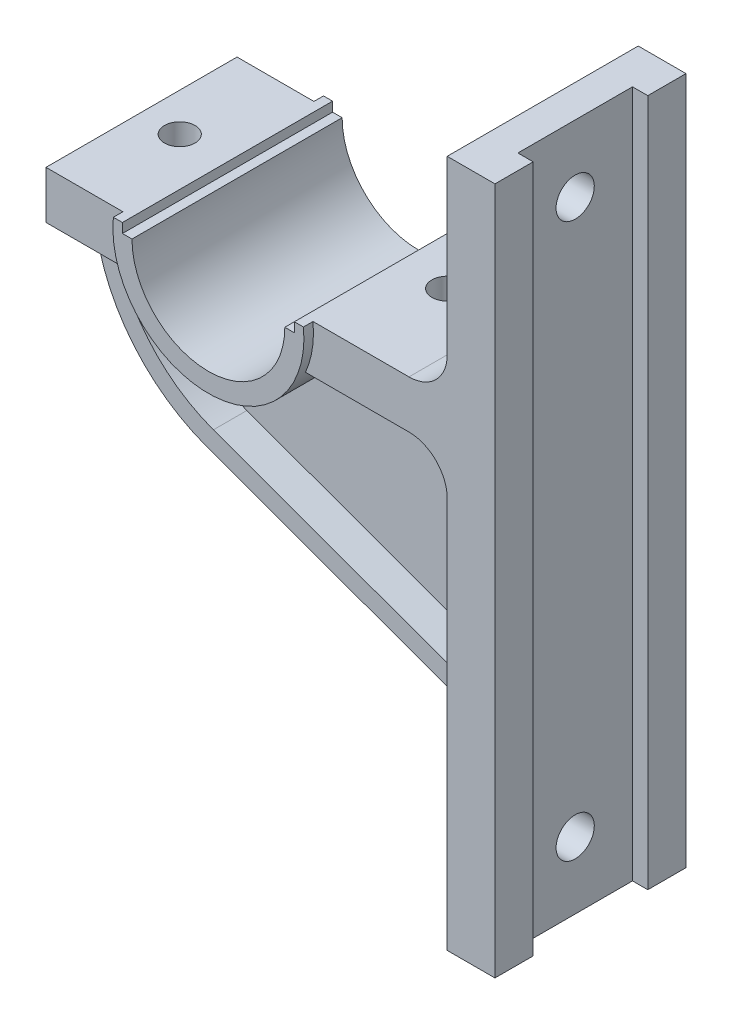
SolidWorks part; units mm, degrees
material "Plain Carbon Steel"
ref_plane "Front Plane" through (0, 0, 0) normal (0, 0, 1) x (1, 0, 0)
ref_plane "Top Plane" through (0, 0, 0) normal (0, 1, 0) x (1, 0, 0)
ref_plane "Right Plane" through (0, 0, 0) normal (1, 0, 0) x (0, 0, -1)
sketch "Bracket Profile Sketch" plane through (0, 0, 0) normal (0, 0, 1) x (1, 0, 0)
  line L0 (-2209.7446, 0) -> (108277.4849, 0) construction
  line L1 (0, -2209.7446) -> (0, 108277.4849) construction
  line L2 (0, 110) -> (0, -250)
  line L3 (0, -250) -> (-25, -250)
  line L4 (-25, -250) -> (-25, -45)
  line L5 (-45, -25) -> (-235, -25)
  line L6 (-235, -25) -> (-235, 0)
  line L7 (-235, 0) -> (-45, 0)
  line L8 (-25, 20) -> (-25, 110)
  line L9 (-25, 110) -> (0, 110)
  arc A0 (-25, -45) -> (-45, -25) centre (-45, -45) ccw
  arc A1 (-45, 0) -> (-25, 20) centre (-45, 20) ccw
  point P16 (-235, -12.5)
  dimension "D4" = 20
  dimension "D5" = 20
  dimension "D1" = 360
  dimension "D2" = 110
  dimension "D3" = 235
  dimension "D6" = 25
  dimension "D7" = 25
  dimension "D8" = 25
extrude "Bracket Body" add sketch "Bracket Profile Sketch" along normal mid plane 100
sketch "Pocket Sketch" plane through (0, 110, 0) normal (0, 1, 0) x (1, 0, 0)
  line L0 (0, -50) -> (0, 50) construction
  line L1 (0, 30) -> (-8, 30)
  line L2 (0, 30) -> (0, -30)
  line L3 (0, -30) -> (-8, -30)
  line L4 (-8, 30) -> (-8, -30)
  dimension "D1" = 60
  dimension "D2" = 30
  dimension "D3" = 8
extrude "Pocket 60x30" cut sketch "Pocket Sketch" against normal through all
sketch "Raised Pad Sketch" plane through (-25, 0, 0) normal (-1, 0, 0) x (0, 0, 1)
  line L0 (0, -1000) -> (0, 49000) construction
  line L1 (50, -250) -> (-50, -250) construction
  circle A0 centre (0, 75) radius 25
  circle A1 centre (0, -215) radius 25
  dimension "D1" = 50
  dimension "D2" = 50
  dimension "D3" = 290
  dimension "D4" = 35
extrude "Raised Pad 5mm" add sketch "Raised Pad Sketch" along normal blind 5
sketch "Pad Hole Sketch" plane through (-30, 0, 0) normal (-1, 0, 0) x (0, 0, 1)
  circle A0 centre (0, 75) radius 10
  circle A1 centre (0, -215) radius 10
  dimension "D1" = 20
  dimension "D2" = 20
extrude "Pad Holes" cut sketch "Pad Hole Sketch" against normal through all
sketch "Mounting Hole Sketch" plane through (0, 0, 0) normal (0, 1, 0) x (1, 0, 0)
  circle A0 centre (-75, 0) radius 7.25
  circle A1 centre (-215, 0) radius 7.25
  dimension "D3" = 14.5
  dimension "D4" = 14.5
  dimension "D1" = 140
  dimension "D2" = 75
extrude "Mounting Holes" cut sketch "Mounting Hole Sketch" against normal blind 25
sketch "Through Hole Sketch" plane through (0, 0, 0) normal (0, 1, 0) x (1, 0, 0)
  circle A0 centre (-75, 0) radius 8
  circle A1 centre (-215, 0) radius 8
  dimension "D1" = 16
  dimension "D2" = 16
extrude "Through Holes Ø16" cut sketch "Through Hole Sketch" against normal blind 20
sketch "Saddle Block Sketch" plane through (0, 0, 0) normal (0, 0, 1) x (1, 0, 0)
  line L0 (-45, 0) -> (-235, 0) construction
  line L2 (-194.7494, 0) -> (-95.2506, 0)
  arc A0 (-194.7494, 0) -> (-95.2506, 0) centre (-145, -5) ccw
  dimension "D2" = 100
  dimension "D1" = 5
  dimension "D3" = 145
extrude "Saddle Block" add sketch "Saddle Block Sketch" along normal mid plane 110
sketch "Pipe Saddle Cut Sketch" plane through (0, 0, 0) normal (0, 0, 1) x (1, 0, 0)
  line L0 (-95.2506, 0) -> (-194.7494, 0) construction
  line L1 (-190, 0) -> (-100, 0)
  line L2 (-190, 0) -> (-190, -5)
  line L3 (-190, -5) -> (-185, -5)
  line L4 (-100, 0) -> (-100, -5)
  line L5 (-105, -5) -> (-100, -5)
  arc A0 (-185, -5) -> (-105, -5) centre (-145, -5) ccw
  point P9 (-190, -2.5)
  dimension "D1" = 80
  dimension "D2" = 5
  dimension "D3" = 90
  dimension "D4" = 45
extrude "Pipe Saddle Cut" cut sketch "Pipe Saddle Cut Sketch" against normal mid plane 110
sketch "Support Arm Sketch" plane through (0, 0, 0) normal (0, 0, 1) x (1, 0, 0)
  line L0 (-41.4495, -158.4653) -> (-175.7818, -109.5723)
  line L1 (-25, -45) -> (-25, -250) construction
  line L2 (-235, 0) -> (-235, -25) construction
  line L3 (-219.8331, -25) -> (-235, -25)
  line L4 (-235, -25) -> (-190.8258, -25) construction
  line L5 (-172.3616, -100.1754) -> (-42.4463, -147.4607)
  line L6 (-25, -181.9576) -> (-25, -135.2447)
  arc A0 (-175.7818, -109.5723) -> (-235, -25) centre (-145, -25) cw
  arc A1 (-25, -181.9576) -> (-41.4495, -158.4653) centre (-50, -181.9576) ccw
  arc A2 (-224.822, -30.3333) -> (-172.3616, -100.1754) centre (-145, -25) ccw
  arc A3 (-42.4463, -147.4607) -> (-25, -135.2447) centre (-38, -135.2447) ccw
  arc A4 (-219.8331, -25) -> (-224.822, -30.3333) centre (-219.8331, -30) ccw
  dimension "D1" = 90
  dimension "D3" = 50
  dimension "D6" = 13
  dimension "D7" = 10
  dimension "D4" = 10
  dimension "D2" = 110
  dimension "D5" = 10
extrude "Support Arm" add sketch "Support Arm Sketch" along normal mid plane 50
sketch "Support Web Sketch" plane through (0, 0, 0) normal (0, 0, 1) x (1, 0, 0)
  line L0 (-25, -45) -> (-25, -135.2447)
  line L1 (-42.4463, -147.4607) -> (-172.3616, -100.1754)
  line L2 (-219.8331, -25) -> (-190.8258, -25)
  line L3 (-45, -25) -> (-99.1742, -25)
  arc A0 (-25, -135.2447) -> (-42.4463, -147.4607) centre (-38, -135.2447) cw
  arc A1 (-42.4463, -147.4607) -> (-25, -135.2447) centre (-38, -135.2447) ccw construction
  arc A2 (-172.3616, -100.1754) -> (-224.822, -30.3333) centre (-145, -25) cw
  arc A3 (-224.822, -30.3333) -> (-219.8331, -25) centre (-219.8331, -30) cw
  arc A4 (-190.8258, -25) -> (-99.1742, -25) centre (-145, -5) ccw
  arc A5 (-25, -45) -> (-45, -25) centre (-45, -45) ccw
extrude "Support Web 15mm" add sketch "Support Web Sketch" along normal mid plane 15
